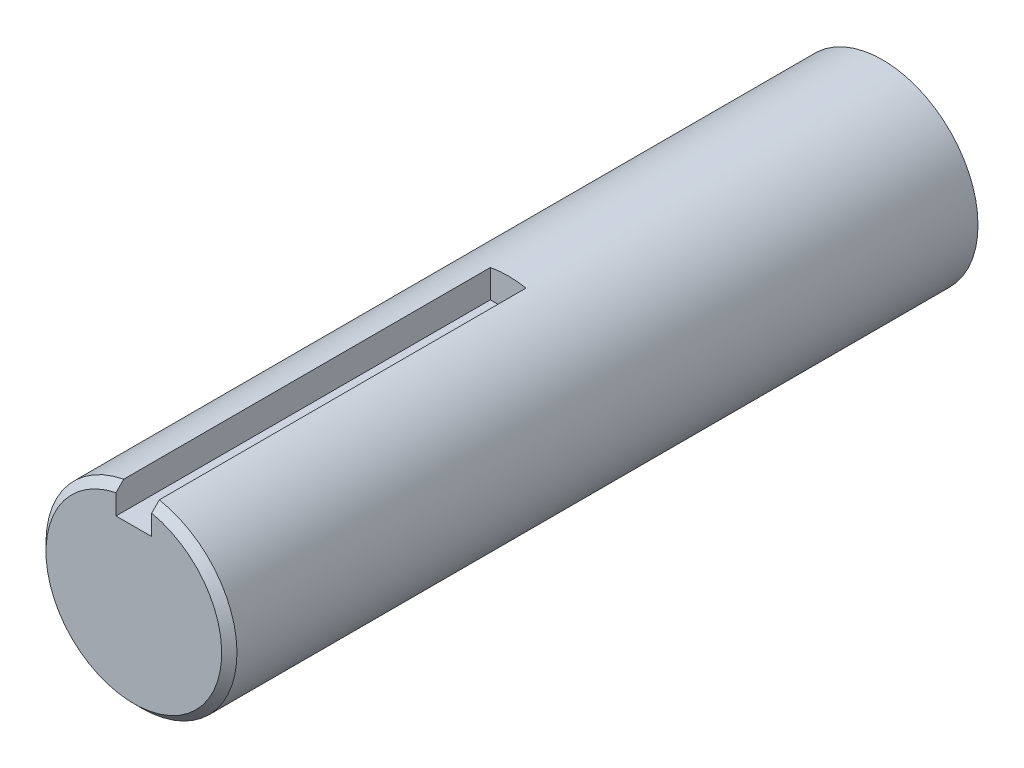
from build123d import *

# Parameters (mm, degrees)
SHAFT_PROFILE_75_R      = 37.5
SHAFT_BODY_75X294_DEPTH = 294
KEYWAY_START            = -147
KEYWAY_CUT_14X147_DEPTH = 147
END_CHAMFER_3X45_SIZE   = 3


with BuildPart() as part:
    # Shaft Profile Ø75 → Shaft Body Ø75x294 (new body)
    with BuildSketch(Plane.XY):
        Circle(SHAFT_PROFILE_75_R)
    extrude(amount=SHAFT_BODY_75X294_DEPTH)

    # Keyway Profile 14 wide → Keyway Cut 14x147 (cut)
    with BuildSketch(Plane.XY.offset(294).offset(KEYWAY_START)):
        with BuildLine():
            Line((-7, 25.84087404), (7, 25.84087404))
            Line((7, 25.84087404), (7, 36.84087404))
            ThreePointArc((7, 36.84087404), (0, 37.5), (-7, 36.84087404))
            Line((-7, 36.84087404), (-7, 25.84087404))
        make_face()
    extrude(amount=KEYWAY_CUT_14X147_DEPTH, mode=Mode.SUBTRACT)

    # End Chamfer 3x45°
    end_chamfer_3x45_edges = [part.edges().sort_by_distance(p)[0] for p in [
        (-23.913908087, -28.885550021, 294),
    ]]
    chamfer(end_chamfer_3x45_edges, length=END_CHAMFER_3X45_SIZE)


solid = part.part
